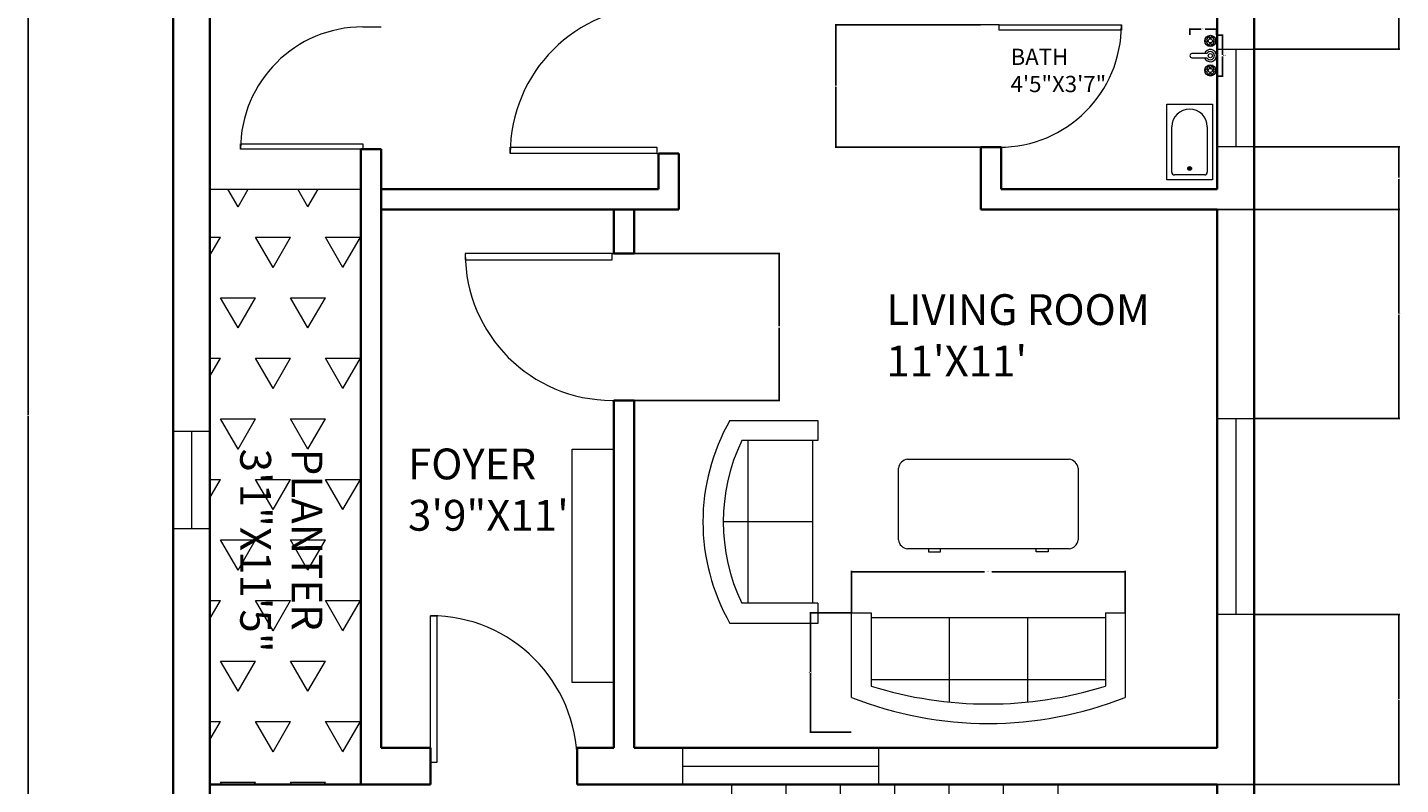
# Model space of a CAD drawing. Units: inches. Extents: x 7766 to 8631, y 9203 to 9940.
# Tile 2 of 6: x 7766 to 8103, y 9510 to 9695. Entities that reach past the tile are written whole.
import ezdxf

# ---------------------------------------------------------------- set-up
doc = ezdxf.new("R2010")
doc.units = ezdxf.units.IN
for name, color, linetype, lineweight in [('A-ANNO-DIMS', 2, 'Continuous', 18), ('A-AREA-IDEN', 11, 'Continuous', 18), ('A-FLOR-FIXT', 9, 'Continuous', 18), ('A-WALL', 7, 'Continuous', 35), ('door', 1, 'Continuous', 18), ('flower', 70, 'Continuous', 18), ('furniture', 6, 'Continuous', 18), ('L-PLNT-PATT', 60, 'Continuous', 13), ('stair', 2, 'Continuous', 18), ('window', 3, 'Continuous', 18)]:
    doc.layers.add(name, color=color, linetype=linetype, lineweight=lineweight)
doc.styles.get("Standard").update_dxf_attribs({"font": 'arial.ttf'})
doc.dimstyles.get("Standard").update_dxf_attribs({"dimtxt": 0.18, "dimasz": 0.18, "dimexe": 0.18, "dimexo": 0.0625, "dimgap": 0.09, "dimtad": 0, "dimtih": 1, "dimtoh": 1, "dimdec": 4, "dimzin": 0, "dimdsep": 46, "dimtxsty": 'Standard', "dimcen": 0.09, "dimadec": 0, "dimazin": 0, "dimtfac": 1, "dimtdec": 4, "dimtofl": 0, "dimtmove": 0, "dimatfit": 3, "dimfxl": 1, "dimtolj": 1, "dimtzin": 0, "dimarcsym": 0})

# ---------------------------------------------------------------- blocks, each defined once
blk = doc.blocks.new('*U3')
for p, q in [((0, 0), (0, -6)), ((-40, 0), (-40, -6))]:
    blk.add_line(p, q)
blk.add_lwpolyline([(0, 0), (0, 40), (-1.75, 40), (-1.75, 0)], close=True)
blk.add_arc((0, 0), 40, 90, 180)
blk = doc.blocks.new('*U2')
for p, q in [((0, 0), (0, -6)), ((40, 0), (40, -6))]:
    blk.add_line(p, q)
blk.add_lwpolyline([(0, 0), (0, 40), (1.75, 40), (1.75, 0)], close=True)
blk.add_arc((0, 0), 40, 0, 90)
blk = doc.blocks.new('*U4')
for p, q in [((0, 0), (0, -6)), ((40, 0), (40, -6))]:
    blk.add_line(p, q)
blk.add_lwpolyline([(0, 0), (0, 40), (1.75, 40), (1.75, 0)], close=True)
blk.add_arc((0, 0), 40, 0, 90)
blk = doc.blocks.new('Desk - 30 x 60 in.')
for p, q in [((-26.999995, 0), (26.999995, 0)), ((-29.999995, -27), (-29.999995, -3)), ((29.999995, -3), (29.999995, -27)), ((26.999995, -30), (-26.999995, -30)), ((-20.000005, -30), (-20.000005, -31)), ((-20.000005, -31), (-16.000005, -31)), ((-16.000005, -31), (-16.000005, -30)), ((15.999995, -31), (15.999995, -30)), ((19.999995, -31), (15.999995, -31)), ((19.999995, -30), (19.999995, -31))]:
    blk.add_line(p, q)
for centre, start, end in [((-26.499995, -3.5), 98.1301, 171.8699), ((26.499995, -3.5), 8.130102, 81.8699), ((-26.499995, -26.5), 188.1301, 261.8699), ((26.499995, -26.5), 278.1301, 351.8699)]:
    blk.add_arc(centre, 3.535534, start, end)
blk = doc.blocks.new('Sofa - Roundback Loveseat 5 ft.')
for p, q in [((0, -32.44198), (0, -5.99998)), ((-24, -33.99998), (-24, -11.46958)), ((24.00004, -33.99998), (24.00004, -11.46958)), ((-23.9998, -13.38178), (23.99986, -13.38178)), ((-24, -32.44198), (24.00004, -32.44198))]:
    blk.add_line(p, q)
for points in [[(-24, -33.99998), (-30, -33.99998), (-30, -7.99998)], [(30.00004, -7.99998), (30.00004, -33.99998), (24.00004, -33.99998)]]:
    blk.add_lwpolyline(points)
for centre, radius, start, end in [((0, -60.24998), 60.24998, 60.13715, 119.8628), ((0, -61.38438), 55.38444, 64.32083, 115.6792)]:
    blk.add_arc(centre, radius, start, end)
blk = doc.blocks.new('Sofa - Roundback 7 ft.')
for p, q in [((-12.00002, -32.4421), (-12.00003, -6.5971)), ((11.99997, -32.4421), (11.99998, -6.5971)), ((-36.000027, -34), (-36.000027, -11.4696)), ((35.99998, -34), (35.99998, -11.4696)), ((-35.999844, -13.3819), (35.9998, -13.3819)), ((-36.000027, -32.4421), (35.99998, -32.4421))]:
    blk.add_line(p, q)
for points in [[(-36.000027, -34), (-42.000027, -34), (-42.000027, -8)], [(41.99998, -8), (41.99998, -34), (35.99998, -34)]]:
    blk.add_lwpolyline(points)
for centre, radius, start, end in [((0, -114.25), 114.25, 68.43141, 111.5686), ((-0.00001, -127.1968), 121.1968, 72.72033, 107.2797)]:
    blk.add_arc(centre, radius, start, end)
blk = doc.blocks.new('Faucet - Bathroom top')
for p, q in [((-4.107, 0.125), (-4.375, 0.125)), ((-3.75, 0.4788), (-3.75, 0.75)), ((-3.5, 0.482), (-3.5, 0.75)), ((-3.1461, 0.125), (-2.875, 0.125)), ((3.143, 0.125), (2.875, 0.125)), ((3.5, 0.4788), (3.5, 0.75)), ((3.75, 0.482), (3.75, 0.75)), ((4.1039, 0.125), (4.375, 0.125)), ((-4.1039, -0.125), (-4.375, -0.125)), ((-3.75, -0.4821), (-3.75, -0.75)), ((-3.5, -0.4789), (-3.5, -0.75)), ((-3.143, -0.125), (-2.875, -0.125)), ((-0.5, -0.8639), (-0.5, -4.5)), ((0.5, -4.5), (0.5, -0.8631)), ((3.1461, -0.125), (2.875, -0.125)), ((3.5, -0.4821), (3.5, -0.75)), ((3.75, -0.4789), (3.75, -0.75)), ((4.107, -0.125), (4.375, -0.125))]:
    blk.add_line(p, q)
for centre, radius in [((-3.625, 0), 1.375), ((-4.625, 0), 0.2795), ((-3.625, 0), 0.5), ((-3.625, 1), 0.2795), ((-2.625, 0), 0.2795), ((0, 0), 0.5), ((3.625, 0), 1.375), ((2.625, 0), 0.2795), ((3.625, 0), 0.5), ((3.625, 1), 0.2795), ((4.625, 0), 0.2795), ((-3.625, -1), 0.2795), ((3.625, -1), 0.2795)]:
    blk.add_circle(centre, radius)
for centre, radius, start, end in [((-3.625, 0), 1, 105.2407, 164.2093), ((-3.625, 0), 1, 16.44125, 74.07887), ((0, 0), 1.5, 289.6514, 250.3603), ((0, 0), 1, 300.3431, 239.7554), ((3.625, 0), 1, 106.12, 164.0884), ((3.625, 0), 1, 16.23422, 73.90469), ((-3.625, 0), 1, 196.2342, 253.9047), ((-3.625, 0), 1, 286.12, 344.0884), ((3.625, 0), 1, 196.4413, 254.0789), ((3.625, 0), 1, 285.2407, 344.2093), ((0, -4.5), 0.5, 180, 0)]:
    blk.add_arc(centre, radius, start, end)
blk = doc.blocks.new('Bath Tub - 26 x 60 in.')
for p, q in [((8, -18), (10, -18)), ((9, -17), (9, -19))]:
    blk.add_line(p, q)
blk.add_lwpolyline([(0, -36), (0, 0), (60, 0), (60, -36)], close=True)
for points in [[(4, -30), (4, -6)], [(6, -4), (42, -4)], [(42, -32), (6, -32)]]:
    blk.add_lwpolyline(points)
for radius in [1.5, 1]:
    blk.add_circle((9, -18), radius)
for centre, radius, start, end in [((5.75, -5.75), 1.77, 81.8699, 188.1301), ((42, -18), 14, 270, 90), ((5.75, -30.25), 1.77, 171.8699, 278.1301)]:
    blk.add_arc(centre, radius, start, end)
blk = doc.blocks.new('WIN-48IN')
blk.add_line((4.5, 48), (4.5, 0))
blk.add_lwpolyline([(0, 48), (9, 48), (9, 0), (0, 0)], close=True)
blk = doc.blocks.new('WIN-24IN')
blk.add_line((4.5, 24), (4.5, 0))
blk.add_lwpolyline([(0, 24), (9, 24), (9, 0), (0, 0)], close=True)
blk = doc.blocks.new('STAIR-U-RETURN')
for p, q in [((8.13, 89), (8.13, 128)), ((21.45, 89), (21.45, 128)), ((34.76, 89), (34.76, 128)), ((48.08, 89), (48.08, 128)), ((61.39, 89), (61.39, 128)), ((74.71, 89), (74.71, 128)), ((88.13, 0), (88.13, 128)), ((0, 107.36), (106.07, 107.36)), ((106.07, 107.36), (106.07, 19.51)), ((13.13, 89), (8.13, 89)), ((13.13, 89), (88.13, 89)), ((88.13, 89), (127.13, 89)), ((88.13, 76.5), (127.13, 76.5)), ((88.13, 64), (127.13, 64)), ((88.13, 51.5), (127.13, 51.5)), ((8.13, 39), (88.13, 39)), ((8.13, 39), (8.13, 0)), ((21.45, 39), (21.45, 0)), ((34.76, 39), (34.76, 0)), ((48.08, 39), (48.08, 0)), ((61.39, 39), (61.39, 0)), ((74.71, 39), (74.71, 0)), ((88.13, 39), (127.13, 39)), ((106.07, 19.51), (8.13, 19.5))]:
    blk.add_line(p, q)
blk = doc.blocks.new('*D44')
at = {"layer": 'A-ANNO-DIMS', "color": 0, "lineweight": -2, "transparency": 16777216}
for p, q in [((7968.54, 9551.75), (7968.54, 9561.93)), ((7968.72, 9561.75), (8001.18, 9561.75)), ((8035.45, 9561.75), (8002.99, 9561.75)), ((8035.63, 9551.75), (8035.63, 9561.93))]:
    blk.add_line(p, q, dxfattribs=at)
at = {"layer": 'A-ANNO-DIMS', "color": 0, "transparency": 16777216}
for points in [[(7968.72, 9561.78), (7968.72, 9561.72), (7968.54, 9561.75)], [(8035.45, 9561.78), (8035.45, 9561.72), (8035.63, 9561.75)]]:
    blk.add_solid(points, dxfattribs=at)
at = {"layer": 'Defpoints', "color": 0, "transparency": 16777216}
for p in [(7968.54, 9561.75), (7968.54, 9551.68), (8035.63, 9551.68)]:
    blk.add_point(p, dxfattribs=at)
at = {"layer": 'A-ANNO-DIMS', "color": 0, "transparency": 16777216, "insert": (8002.09, 9561.75), "char_height": 0.18, "attachment_point": 5}
blk.add_mtext('\\A1;SOFA 67 TYP.', dxfattribs=at)
blk = doc.blocks.new('*D45')
at = {"layer": 'A-ANNO-DIMS', "color": 0, "lineweight": -2, "transparency": 16777216}
for p, q in [((7968.48, 9551.68), (7958.3, 9551.68)), ((7958.48, 9551.5), (7958.48, 9537.22)), ((7958.48, 9522.58), (7958.48, 9536.86)), ((7968.48, 9522.4), (7958.3, 9522.4))]:
    blk.add_line(p, q, dxfattribs=at)
at = {"layer": 'A-ANNO-DIMS', "color": 0, "transparency": 16777216}
for points in [[(7958.45, 9551.5), (7958.51, 9551.5), (7958.48, 9551.68)], [(7958.45, 9522.58), (7958.51, 9522.58), (7958.48, 9522.4)]]:
    blk.add_solid(points, dxfattribs=at)
at = {"layer": 'Defpoints', "color": 0, "transparency": 16777216}
for p in [(7968.54, 9551.68), (7958.48, 9522.4), (7968.54, 9522.4)]:
    blk.add_point(p, dxfattribs=at)
at = {"layer": 'A-ANNO-DIMS', "color": 0, "transparency": 16777216, "insert": (7958.48, 9537.04), "char_height": 0.18, "attachment_point": 5}
blk.add_mtext('\\A1;29 TYP.', dxfattribs=at)
blk = doc.blocks.new('*D54')
at = {"layer": 'A-ANNO-DIMS', "color": 0, "lineweight": -2, "transparency": 16777216}
for p, q in [((8058.09, 9693.31), (8059.71, 9693.31)), ((8059.53, 9693.13), (8059.53, 9688.49)), ((8059.53, 9683.49), (8059.53, 9688.12)), ((8058.09, 9683.31), (8059.71, 9683.31))]:
    blk.add_line(p, q, dxfattribs=at)
at = {"layer": 'A-ANNO-DIMS', "color": 0, "transparency": 16777216}
for points in [[(8059.5, 9693.13), (8059.56, 9693.13), (8059.53, 9693.31)], [(8059.5, 9683.49), (8059.56, 9683.49), (8059.53, 9683.31)]]:
    blk.add_solid(points, dxfattribs=at)
at = {"layer": 'Defpoints', "color": 0, "transparency": 16777216}
for p in [(8058.03, 9693.31), (8058.03, 9683.31), (8059.53, 9683.31)]:
    blk.add_point(p, dxfattribs=at)
at = {"layer": 'A-ANNO-DIMS', "color": 0, "transparency": 16777216, "insert": (8059.53, 9688.31), "char_height": 0.18, "attachment_point": 5}
blk.add_mtext('\\A1;FAUCET 10 TYP.', dxfattribs=at)
blk = doc.blocks.new('*D55')
at = {"layer": 'A-ANNO-DIMS', "color": 0, "lineweight": -2, "transparency": 16777216}
for p, q in [((8051.53, 9693.37), (8051.53, 9694.99)), ((8051.71, 9694.81), (8054.32, 9694.81)), ((8057.85, 9694.81), (8055.24, 9694.81)), ((8058.03, 9693.37), (8058.03, 9694.99))]:
    blk.add_line(p, q, dxfattribs=at)
at = {"layer": 'A-ANNO-DIMS', "color": 0, "transparency": 16777216}
for points in [[(8051.71, 9694.84), (8051.71, 9694.78), (8051.53, 9694.81)], [(8057.85, 9694.84), (8057.85, 9694.78), (8058.03, 9694.81)]]:
    blk.add_solid(points, dxfattribs=at)
at = {"layer": 'Defpoints', "color": 0, "transparency": 16777216}
for p in [(8051.53, 9693.31), (8058.03, 9694.81), (8058.03, 9693.31)]:
    blk.add_point(p, dxfattribs=at)
at = {"layer": 'A-ANNO-DIMS', "color": 0, "transparency": 16777216, "insert": (8054.78, 9694.81), "char_height": 0.18, "attachment_point": 5}
blk.add_mtext('\\A1;7 TYP.', dxfattribs=at)
blk = doc.blocks.new('*D69')
at = {"layer": 'A-ANNO-DIMS', "color": 0, "lineweight": -2, "transparency": 16777216}
for p, q in [((7802.18, 9904.56), (7766.51, 9904.56)), ((7766.69, 9904.38), (7766.69, 9600.25)), ((7766.69, 9295.74), (7766.69, 9599.88)), ((7802.18, 9295.56), (7766.51, 9295.56))]:
    blk.add_line(p, q, dxfattribs=at)
at = {"layer": 'A-ANNO-DIMS', "color": 0, "transparency": 16777216}
for points in [[(7766.66, 9904.38), (7766.72, 9904.38), (7766.69, 9904.56)], [(7766.66, 9295.74), (7766.72, 9295.74), (7766.69, 9295.56)]]:
    blk.add_solid(points, dxfattribs=at)
at = {"layer": 'Defpoints', "color": 0, "transparency": 16777216}
for p in [(7766.69, 9904.56), (7802.24, 9904.56), (7802.24, 9295.56)]:
    blk.add_point(p, dxfattribs=at)
at = {"layer": 'A-ANNO-DIMS', "color": 0, "transparency": 16777216, "insert": (7766.69, 9600.06), "char_height": 0.18, "attachment_point": 5}
blk.add_mtext('\\A1;609', dxfattribs=at)
blk = doc.blocks.new('*D81')
at = {"layer": 'A-ANNO-DIMS', "color": 0, "lineweight": -2, "transparency": 16777216}
for p, q in [((8067.31, 9551.3), (8102.97, 9551.3)), ((8102.79, 9551.12), (8102.79, 9530.61)), ((8102.79, 9509.74), (8102.79, 9530.25)), ((8058.31, 9509.56), (8102.97, 9509.56))]:
    blk.add_line(p, q, dxfattribs=at)
at = {"layer": 'A-ANNO-DIMS', "color": 0, "transparency": 16777216}
for points in [[(8102.76, 9551.12), (8102.82, 9551.12), (8102.79, 9551.3)], [(8102.76, 9509.74), (8102.82, 9509.74), (8102.79, 9509.56)]]:
    blk.add_solid(points, dxfattribs=at)
at = {"layer": 'Defpoints', "color": 0, "transparency": 16777216}
for p in [(8067.24, 9551.3), (8102.79, 9551.3), (8058.24, 9509.56)]:
    blk.add_point(p, dxfattribs=at)
at = {"layer": 'A-ANNO-DIMS', "color": 0, "transparency": 16777216, "insert": (8102.79, 9530.43), "char_height": 0.18, "attachment_point": 5}
blk.add_mtext('\\A1;41.73', dxfattribs=at)
blk = doc.blocks.new('*D82')
at = {"layer": 'A-ANNO-DIMS', "color": 0, "lineweight": -2, "transparency": 16777216}
for p, q in [((8058.31, 9650.56), (8102.97, 9650.56)), ((8102.79, 9650.38), (8102.79, 9625.11)), ((8102.79, 9599.48), (8102.79, 9624.75)), ((8067.31, 9599.3), (8102.97, 9599.3))]:
    blk.add_line(p, q, dxfattribs=at)
at = {"layer": 'A-ANNO-DIMS', "color": 0, "transparency": 16777216}
for points in [[(8102.76, 9650.38), (8102.82, 9650.38), (8102.79, 9650.56)], [(8102.76, 9599.48), (8102.82, 9599.48), (8102.79, 9599.3)]]:
    blk.add_solid(points, dxfattribs=at)
at = {"layer": 'Defpoints', "color": 0, "transparency": 16777216}
for p in [(8058.24, 9650.56), (8102.79, 9650.56), (8067.24, 9599.3)]:
    blk.add_point(p, dxfattribs=at)
at = {"layer": 'A-ANNO-DIMS', "color": 0, "transparency": 16777216, "insert": (8102.79, 9624.93), "char_height": 0.18, "attachment_point": 5}
blk.add_mtext('\\A1;51.27', dxfattribs=at)
blk = doc.blocks.new('*D83')
at = {"layer": 'A-ANNO-DIMS', "color": 0, "lineweight": -2, "transparency": 16777216}
for p, q in [((8067.31, 9665.91), (8102.97, 9665.91)), ((8102.79, 9665.73), (8102.79, 9658.42)), ((8102.79, 9650.74), (8102.79, 9658.05)), ((8058.31, 9650.56), (8102.97, 9650.56))]:
    blk.add_line(p, q, dxfattribs=at)
at = {"layer": 'A-ANNO-DIMS', "color": 0, "transparency": 16777216}
for points in [[(8102.76, 9665.73), (8102.82, 9665.73), (8102.79, 9665.91)], [(8102.76, 9650.74), (8102.82, 9650.74), (8102.79, 9650.56)]]:
    blk.add_solid(points, dxfattribs=at)
at = {"layer": 'Defpoints', "color": 0, "transparency": 16777216}
for p in [(8067.24, 9665.91), (8102.79, 9665.91), (8058.24, 9650.56)]:
    blk.add_point(p, dxfattribs=at)
at = {"layer": 'A-ANNO-DIMS', "color": 0, "transparency": 16777216, "insert": (8102.79, 9658.24), "char_height": 0.18, "attachment_point": 5}
blk.add_mtext('\\A1;15.347', dxfattribs=at)
blk = doc.blocks.new('*D84')
at = {"layer": 'A-ANNO-DIMS', "color": 0, "lineweight": -2, "transparency": 16777216}
for p, q in [((8067.31, 9736.18), (8102.97, 9736.18)), ((8102.79, 9736), (8102.79, 9713.23)), ((8102.79, 9690.09), (8102.79, 9712.86)), ((8067.31, 9689.91), (8102.97, 9689.91))]:
    blk.add_line(p, q, dxfattribs=at)
at = {"layer": 'A-ANNO-DIMS', "color": 0, "transparency": 16777216}
for points in [[(8102.76, 9736), (8102.82, 9736), (8102.79, 9736.18)], [(8102.76, 9690.09), (8102.82, 9690.09), (8102.79, 9689.91)]]:
    blk.add_solid(points, dxfattribs=at)
at = {"layer": 'Defpoints', "color": 0, "transparency": 16777216}
for p in [(8067.24, 9736.18), (8102.79, 9736.18), (8067.24, 9689.91)]:
    blk.add_point(p, dxfattribs=at)
at = {"layer": 'A-ANNO-DIMS', "color": 0, "transparency": 16777216, "insert": (8102.79, 9713.05), "char_height": 0.18, "attachment_point": 5}
blk.add_mtext('\\A1;46.27', dxfattribs=at)
blk = doc.blocks.new('*D93')
at = {"layer": 'A-ANNO-DIMS', "color": 0, "lineweight": -2, "transparency": 16777216}
for p, q in [((8000.18, 9695.83), (7964.51, 9695.83)), ((7964.69, 9695.65), (7964.69, 9681.01)), ((7964.69, 9666.01), (7964.69, 9680.65)), ((8000.18, 9665.83), (7964.51, 9665.83))]:
    blk.add_line(p, q, dxfattribs=at)
at = {"layer": 'A-ANNO-DIMS', "color": 0, "transparency": 16777216}
for points in [[(7964.66, 9695.65), (7964.72, 9695.65), (7964.69, 9695.83)], [(7964.66, 9666.01), (7964.72, 9666.01), (7964.69, 9665.83)]]:
    blk.add_solid(points, dxfattribs=at)
at = {"layer": 'Defpoints', "color": 0, "transparency": 16777216}
for p in [(7964.69, 9695.83), (8000.24, 9695.83), (8000.24, 9665.83)]:
    blk.add_point(p, dxfattribs=at)
at = {"layer": 'A-ANNO-DIMS', "color": 0, "transparency": 16777216, "insert": (7964.69, 9680.83), "char_height": 0.18, "attachment_point": 5}
blk.add_mtext('\\A1;30', dxfattribs=at)
blk = doc.blocks.new('*D100')
at = {"layer": 'A-ANNO-DIMS', "color": 0, "lineweight": -2, "transparency": 16777216}
for p, q in [((7915.31, 9639.78), (7950.97, 9639.78)), ((7950.79, 9639.6), (7950.79, 9621.96)), ((7950.79, 9603.96), (7950.79, 9621.6)), ((7915.31, 9603.78), (7950.97, 9603.78))]:
    blk.add_line(p, q, dxfattribs=at)
at = {"layer": 'A-ANNO-DIMS', "color": 0, "transparency": 16777216}
for points in [[(7950.76, 9639.6), (7950.82, 9639.6), (7950.79, 9639.78)], [(7950.76, 9603.96), (7950.82, 9603.96), (7950.79, 9603.78)]]:
    blk.add_solid(points, dxfattribs=at)
at = {"layer": 'Defpoints', "color": 0, "transparency": 16777216}
for p in [(7915.24, 9639.78), (7915.24, 9603.78), (7950.79, 9603.78)]:
    blk.add_point(p, dxfattribs=at)
at = {"layer": 'A-ANNO-DIMS', "color": 0, "transparency": 16777216, "insert": (7950.79, 9621.78), "char_height": 0.18, "attachment_point": 5}
blk.add_mtext('\\A1;36', dxfattribs=at)

msp = doc.modelspace()

# ---------------------------------------------------------------- hatches: boundary and pattern name
at = {"layer": 'L-PLNT-PATT'}
h = msp.add_hatch(dxfattribs=at)
h.set_pattern_fill('TRIANG', color=256, scale=1.8)
h.paths.add_polyline_path([(7848.243, 9895.5631), (7811.243, 9895.5631), (7811.243, 9784.5631), (7848.243, 9784.5631)])
h.paths.add_polyline_path([(7848.243, 9655.5631), (7811.243, 9655.5631), (7811.243, 9509.5631), (7848.243, 9509.5631)])
h.paths.add_polyline_path([(8058.243, 9372.5631), (7939.243, 9372.5631), (7939.243, 9304.5631), (8058.243, 9304.5631)])
h.paths.add_polyline_path([(7817.6934, 9855.8718), (7817.6934, 9803.4053), (7845.8896, 9803.4053), (7845.8896, 9855.8718)], flags=24)
h.paths.add_polyline_path([(7814.5059, 9594.625), (7814.5059, 9542.1584), (7842.7021, 9542.1584), (7842.7021, 9594.625)], flags=24)
h.paths.add_polyline_path([(7965.0141, 9329.808), (8013.9551, 9329.808), (8013.9551, 9358.0042), (7965.0141, 9358.0042)], flags=24)

# ---------------------------------------------------------------- linework, layer by layer
at = {"layer": 'A-WALL'}
for p, q in [((7802.243, 9295.5631), (7802.243, 9904.5631)), ((7811.243, 9509.5631), (7811.243, 9895.5631)), ((8067.243, 9895.5631), (8067.243, 9295.5631)), ((8058.243, 9655.5631), (8058.243, 9698.5631)), ((7848.243, 9509.5631), (7848.243, 9665.3613)), ((7853.243, 9518.5631), (7853.243, 9665.3613)), ((7921.243, 9655.5631), (7921.243, 9664.3108)), ((7926.243, 9650.5631), (7926.243, 9664.3108)), ((8000.243, 9650.5631), (8000.243, 9665.831)), ((8005.243, 9655.5631), (8005.243, 9665.831)), ((7853.243, 9655.5631), (7921.243, 9655.5631)), ((7853.243, 9655.5631), (7921.243, 9655.5631)), ((8005.243, 9655.5631), (8058.243, 9655.5631)), ((7853.243, 9650.5631), (7926.243, 9650.5631)), ((7910.243, 9639.7799), (7910.243, 9650.5631)), ((7915.243, 9639.7799), (7915.243, 9650.5631)), ((8000.243, 9650.5631), (8058.243, 9650.5631)), ((8058.243, 9518.5631), (8058.243, 9650.5631)), ((7910.243, 9518.5631), (7910.243, 9603.7799)), ((7915.243, 9518.5631), (7915.243, 9603.7799)), ((7853.243, 9518.5631), (7865.2947, 9518.5631)), ((7901.2947, 9518.5631), (7910.243, 9518.5631)), ((7915.243, 9518.5631), (7944.243, 9518.5631)), ((7939.243, 9518.5631), (7944.243, 9518.5631)), ((7944.243, 9518.5631), (8058.243, 9518.5631)), ((7811.243, 9304.5631), (7811.243, 9509.5631)), ((7811.243, 9509.5631), (7865.2947, 9509.5631)), ((7901.2947, 9509.5631), (7944.243, 9509.5631)), ((7939.243, 9509.5631), (7944.243, 9509.5631)), ((7944.243, 9509.5631), (8058.243, 9509.5631)), ((8058.243, 9381.5631), (8058.243, 9509.5631))]:
    msp.add_line(p, q, dxfattribs=at)
for points in [[(7853.243, 9665.3613), (7848.243, 9665.3613)], [(7926.243, 9664.3108), (7921.243, 9664.3108)], [(8005.243, 9665.831), (8000.243, 9665.831)], [(7910.243, 9639.7799), (7915.243, 9639.7799)], [(7915.243, 9603.7799), (7910.243, 9603.7799)], [(7865.2947, 9509.5631), (7865.2947, 9518.5631)], [(7901.2947, 9518.5631), (7901.2947, 9509.5631)]]:
    msp.add_lwpolyline(points, dxfattribs=at)
at = {"layer": 'flower'}
msp.add_line((7811.243, 9655.5631), (7848.243, 9655.5631), dxfattribs=at)
msp.add_lwpolyline([(7811.243, 9655.5631), (7848.243, 9655.5631), (7848.243, 9509.5631), (7811.243, 9509.5631)], close=True, dxfattribs=at)
at = {"layer": 'furniture'}
msp.add_lwpolyline([(7900.0522, 9591.8126), (7910.243, 9591.8126), (7910.243, 9534.5667), (7900.0522, 9534.5667)], close=True, dxfattribs=at)

# ---------------------------------------------------------------- block references
at = {"layer": 'A-FLOR-FIXT', "rotation": 270}
msp.add_blockref('Faucet - Bathroom top', (8056.53, 9688.3072), dxfattribs=at)
at = {"layer": 'A-FLOR-FIXT', "xscale": 0.3098883198950951, "yscale": 0.3098883198950951, "zscale": 0.3098883198950951, "rotation": 90}
msp.add_blockref('Bath Tub - 26 x 60 in.', (8045.8668, 9657.8539), dxfattribs=at)
at = {"layer": 'door'}
for name, p, xscale, yscale, zscale, rotation in [('*U4', (7920.843, 9664.3108), 0.9, 0.9, 0.9, 90), ('*U2', (7848.743, 9665.3613), 0.75, 0.75, 0.75, 90), ('*U2', (8004.743, 9695.831), 0.75, 0.75, 0.75, 270), ('*U3', (7909.843, 9639.7799), 0.9, 0.9, 0.9, 90)]:
    msp.add_blockref(name, p, dxfattribs=dict(at, xscale=xscale, yscale=yscale, zscale=zscale, rotation=rotation))
at = {"layer": 'door', "xscale": 0.9, "yscale": 0.9, "zscale": 0.9}
msp.add_blockref('*U2', (7865.2947, 9514.9631), dxfattribs=at)
at = {"layer": 'furniture'}
for name, p, xscale, yscale, zscale, rotation in [('Sofa - Roundback Loveseat 5 ft.', (7932.1088, 9573.9784), 0.829764444386874, 0.829764444386874, 0.829764444386874, 90), ('Sofa - Roundback 7 ft.', (8002.0875, 9524.5295), 0.7986556834992792, 0.7986556834992792, 0.7986556834992792, 180)]:
    msp.add_blockref(name, p, dxfattribs=dict(at, xscale=xscale, yscale=yscale, zscale=zscale, rotation=rotation))
at = {"layer": 'furniture', "xscale": 0.7346827235755428, "yscale": 0.7346827235755428, "zscale": 0.7346827235755428}
msp.add_blockref('Desk - 30 x 60 in.', (8002.0875, 9589.3674), dxfattribs=at)
at = {"layer": 'stair'}
msp.add_blockref('STAIR-U-RETURN', (7931.11, 9381.563), dxfattribs=at)
at = {"layer": 'window'}
for name, p in [('WIN-24IN', (8058.243, 9665.9094)), ('WIN-48IN', (8058.243, 9551.2965)), ('WIN-24IN', (7802.243, 9572.2351))]:
    msp.add_blockref(name, p, dxfattribs=at)
at = {"layer": 'window', "rotation": 89.99999999999783}
msp.add_blockref('WIN-48IN', (7975.1963, 9509.5631), dxfattribs=at)

# ---------------------------------------------------------------- texts
at = {"layer": 'A-AREA-IDEN', "attachment_point": 1}
for s, insert, char_height in [('BATH\\P4\'5"X3\'7"', (8007.552, 9690.019), 4), ("LIVING ROOM\\P11'X11'", (7977.0749, 9629.8043), 7.556341), ('FOYER\\P3\'9"X11\'', (7859.8062, 9591.9622), 7.55634)]:
    msp.add_mtext_dynamic_manual_height_columns(s, width=97.347002, gutter_width=18.8909, heights=[0], dxfattribs=dict(at, insert=insert, char_height=char_height))
at = {"layer": 'A-AREA-IDEN', "insert": (7838.8132, 9591.9215), "char_height": 7.55634, "attachment_point": 1, "rotation": 270}
msp.add_mtext_dynamic_manual_height_columns('PLANTER\\P3\'1"X11\'5"', width=97.347002, gutter_width=18.8909, heights=[0], dxfattribs=at)

# ---------------------------------------------------------------- dimensions: what is measured, and where the dimension line sits
at = {"layer": 'A-ANNO-DIMS'}
for base, p1, p2, angle, override, picture, middle in [((7766.693, 9904.5631), (7802.243, 9295.5631), (7802.243, 9904.5631), 90, {"dimdec": 0, "dimlfac": 1, "dimrnd": 0, "dimzin": 0, "dimdsep": 46, "dimlunit": 2}, '*D69', (7766.693, 9600.0631)), ((8102.793, 9736.1825), (8067.243, 9689.9099), (8067.243, 9736.1825), 90, {"dimdec": 2, "dimlfac": 1, "dimrnd": 0, "dimzin": 0, "dimdsep": 46, "dimlunit": 2}, '*D84', (8102.793, 9713.0462)), ((7964.693, 9695.831), (8000.243, 9665.831), (8000.243, 9695.831), 90, {"dimdec": 0, "dimlfac": 1, "dimrnd": 0, "dimzin": 0, "dimdsep": 46, "dimlunit": 2}, '*D93', (7964.693, 9680.831)), ((8102.793, 9665.9099), (8058.243, 9650.5631), (8067.243, 9665.9099), 90, {"dimdec": 3, "dimlfac": 1, "dimrnd": 0, "dimzin": 0, "dimdsep": 46, "dimlunit": 2}, '*D83', (8102.793, 9658.2365)), ((8102.793, 9650.5631), (8067.243, 9599.2962), (8058.243, 9650.5631), 90, {"dimdec": 2, "dimlfac": 1, "dimrnd": 0, "dimzin": 0, "dimdsep": 46, "dimlunit": 2}, '*D82', (8102.793, 9624.9296)), ((7950.793, 9603.7799), (7915.243, 9639.7799), (7915.243, 9603.7799), 270, {"dimdec": 0, "dimlfac": 1, "dimrnd": 0, "dimzin": 0, "dimdsep": 46, "dimlunit": 2}, '*D100', (7950.793, 9621.7799)), ((8102.793, 9551.2962), (8058.243, 9509.5631), (8067.243, 9551.2962), 90, {"dimdec": 2, "dimlfac": 1, "dimrnd": 0, "dimzin": 0, "dimdsep": 46, "dimlunit": 2}, '*D81', (8102.793, 9530.4296))]:
    dim = msp.add_linear_dim(base=base, p1=p1, p2=p2, angle=angle, dimstyle='Standard', override=override, dxfattribs=at)
    dim.commit()
    dim.dimension.update_dxf_attribs({"geometry": picture, "text_midpoint": middle})
dim = msp.add_linear_dim(base=(8058.0301, 9694.8072), p1=(8051.53, 9693.3072), p2=(8058.0301, 9693.3072), text='<> TYP.', dimstyle='Standard', override={"dimdec": 0, "dimlfac": 1, "dimrnd": 0, "dimzin": 0, "dimdsep": 46, "dimlunit": 2}, dxfattribs=at)
dim.commit()
dim.dimension.update_dxf_attribs({"geometry": '*D55', "text_midpoint": (8054.78, 9694.8072)})
for base, p1, p2, angle, text, picture, middle in [((8059.5301, 9683.3072), (8058.0301, 9693.3072), (8058.0301, 9683.3072), 270, 'FAUCET <> TYP.', '*D54', (8059.5301, 9688.3072)), ((7968.544, 9561.7468), (8035.6311, 9551.6838), (7968.544, 9551.6838), 180, 'SOFA <> TYP.', '*D44', (8002.0875, 9561.7468)), ((7958.4809, 9522.3997), (7968.544, 9551.6838), (7968.544, 9522.3997), 270, '<> TYP.', '*D45', (7958.4809, 9537.0418))]:
    dim = msp.add_linear_dim(base=base, p1=p1, p2=p2, angle=angle, text=text, dimstyle='Standard', override={"dimdec": 0, "dimlfac": 1, "dimrnd": 0, "dimzin": 0, "dimdsep": 46, "dimlunit": 2}, dxfattribs=at)
    dim.commit()
    dim.dimension.update_dxf_attribs({"geometry": picture, "text_midpoint": middle})

doc.saveas('drawing.dxf')
